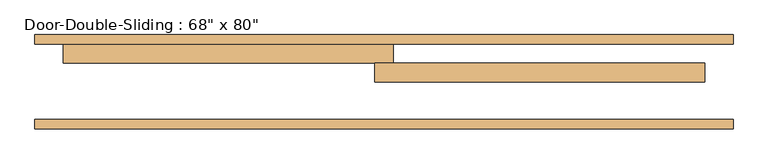
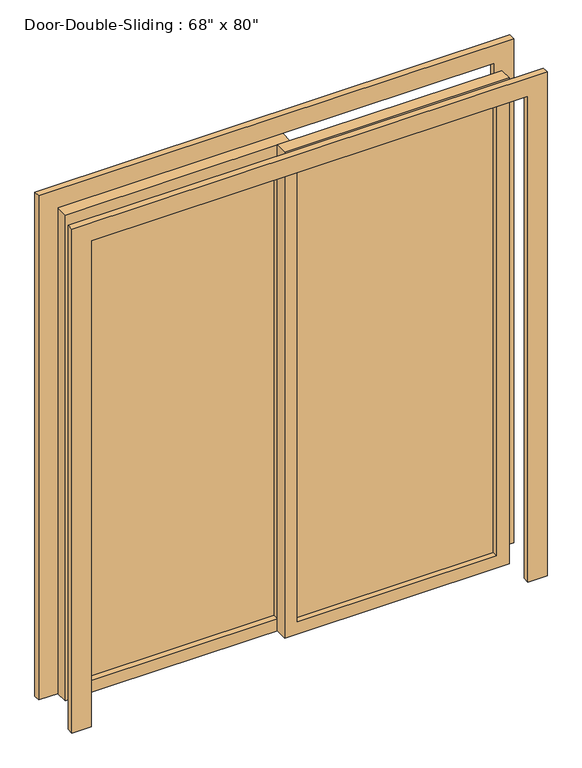
"""IFC4 building model written with IfcOpenShell, lengths in millimetres: door geometry."""

from ifc_helpers import new_model, si_unit, frame, origin, place, context, project, spatial, polyline, outline, extrude, source, transform, mapped, element, save


def door_076b30e0(model_context):
    return source(origin(), model_context, "Body", "SweptSolid", [
        extrude(outline(polyline([(0.0, -939.8), (0.0, -863.6), (2032.0, -863.6), (2032.0, 863.6), (0.0, 863.6), (0.0, 939.8), (2108.2, 939.8), (2108.2, -939.8), (0.0, -939.8)])), frame((0.0, 0.0, 0.0), z_axis=(0.0, 1.0, 0.0), x_axis=(0.0, 0.0, 1.0)), (0.0, 0.0, 1.0), 25.4),
        extrude(outline(polyline([(0.0, 939.8), (2108.2, 939.8), (2108.2, -939.8), (0.0, -939.8), (0.0, -863.6), (2032.0, -863.6), (2032.0, 863.6), (0.0, 863.6), (0.0, 939.8)])), frame((0.0, 228.6, 0.0), z_axis=(0.0, 1.0, 0.0), x_axis=(0.0, 0.0, 1.0)), (0.0, 0.0, 1.0), 25.4),
        extrude(outline(polyline([(2032.0, -25.4), (0.0, -25.4), (0.0, 863.6), (2032.0, 863.6), (2032.0, -25.4)]), holes=[polyline([(1981.2, 25.4), (1981.2, 812.8), (50.8, 812.8), (50.8, 25.4), (1981.2, 25.4)])]), frame((0.0, 127.0, 0.0), z_axis=(0.0, 1.0, 0.0), x_axis=(0.0, 0.0, 1.0)), (0.0, 0.0, 1.0), 50.8),
        extrude(outline(polyline([(2032.0, 25.4), (2032.0, -863.6), (0.0, -863.6), (0.0, 25.4), (2032.0, 25.4)]), holes=[polyline([(1981.2, -25.4), (50.8, -25.4), (50.8, -812.8), (1981.2, -812.8), (1981.2, -25.4)])]), frame((0.0, 177.8, 0.0), z_axis=(0.0, 1.0, 0.0), x_axis=(0.0, 0.0, 1.0)), (0.0, 0.0, 1.0), 50.8),
        extrude(outline(polyline([(25.4, 155.575), (812.8, 155.575), (812.8, 149.225), (25.4, 149.225), (25.4, 155.575)])), frame((0.0, 0.0, 50.8), z_axis=(0.0, 0.0, 1.0), x_axis=(1.0, 0.0, 0.0)), (0.0, 0.0, 1.0), 1930.4),
        extrude(outline(polyline([(-25.4, 200.025), (-812.8, 200.025), (-812.8, 206.375), (-25.4, 206.375), (-25.4, 200.025)])), frame((0.0, 0.0, 50.8), z_axis=(0.0, 0.0, 1.0), x_axis=(1.0, 0.0, 0.0)), (0.0, 0.0, 1.0), 1930.4),
    ])


if __name__ == "__main__":
    model = new_model("IFC4")
    model_context = context("Model", 3, world=origin())
    ifc_project = project(units=[si_unit("LENGTHUNIT", "METRE", prefix="MILLI")], contexts=[model_context])
    site = spatial("IfcSite", under=ifc_project)
    building = spatial("IfcBuilding", under=site)
    placement = place(None, origin())
    door_shape = door_076b30e0(model_context)
    element("IfcDoor", 1, ObjectType="Door-Double-Sliding : 68\" x 80\"", at=placement, inside=building, context=model_context, shape_type="MappedRepresentation", body=[
        mapped(door_shape, transform((0.0, 0.0, 0.0), x_axis=(1.0, 0.0, 0.0), y_axis=(0.0, 1.0, 0.0), z_axis=(0.0, 0.0, 1.0))),
    ])
    save(model, "model.ifc")

# Revit data of these elements
# Type "Door-Double-Sliding : 68\" x 80\""
#   Type Mark = "9"
#   Construction Type Id = "opn-d45"
#   Assembly Code = "C1020"
#   Analytic Construction = "Wood frame, double glass door "
#   Thickness = 0' - 2"
#   Thermal Resistance (R) = 1.8150 (h·ft²·°F)/BTU
#   Heat Transfer Coefficient (U) = 0.5510 BTU/(h·ft²·°F)
#   Height = 6' - 8"
#   Rail Width = 0' - 2"
#   Stiles = 0' - 2"
#   Trim Projection Ext = 0' - 1"
#   Trim Projection Int = 0' - 1"
#   Trim Width = 0' - 3"
#   Width = 5' - 8"
#   Define Thermal Properties by = 1
#   Glazing = Glass
#   Panel Material = Wood - Birch - Solid Stained Light Low Gloss
#   Trim Material = Paint - Sienna
#   Visual Light Transmittance = 0
#   Solar Heat Gain Coefficient = 0
#   Function = (empty or 0)
#   Wall Closure = (empty or 0)
# Element 1 (IfcDoor, "Door-Double-Sliding : 68\" x 80\"")
#   Materials on its faces: "Paint - Sienna", "Wood - Birch - Solid Stained Light Low Gloss", "Glass"
# Materials
#   "Glass": class "Glass", colour RGB 0 128 192, transparency 0.75, Description = "Soda Lime Glass", Cost = 0
#   "Wood - Birch - Solid Stained Light Low Gloss": class "Wood", colour RGB 210 159 95, transparency 0, Cost = 0
#   "Paint - Sienna": colour RGB 118 70 51, transparency 0, Cost = 0
